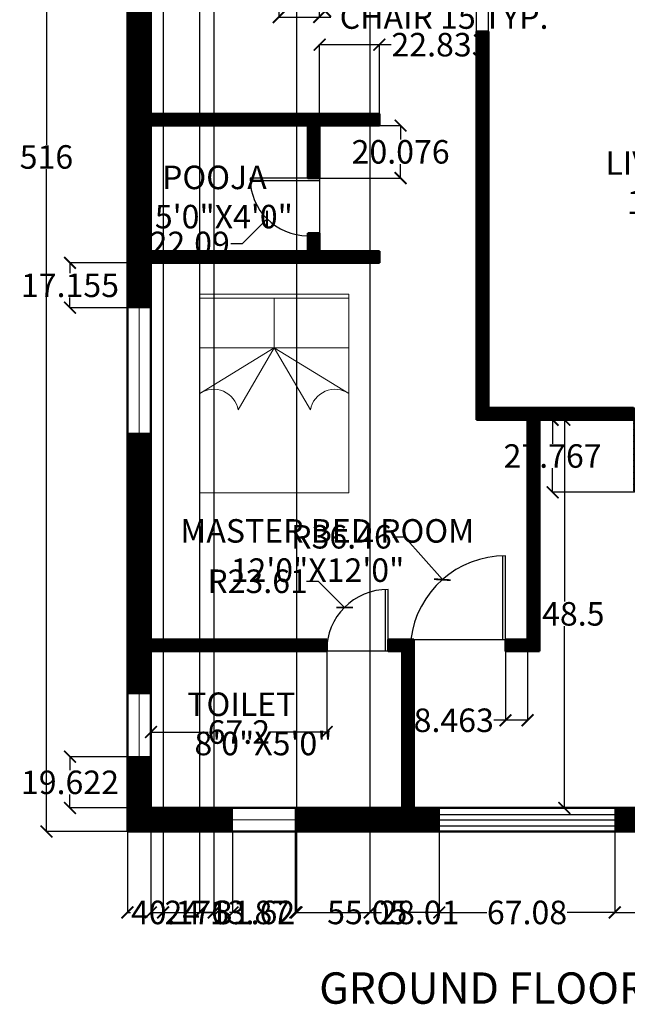
# Model space of a CAD drawing. Units: inches. Extents: x 91 to 526, y 242 to 861.
# Tile 1 of 5: x 96 to 328, y 242 to 618. Entities that reach past the tile are written whole.
import ezdxf

# ---------------------------------------------------------------- set-up
doc = ezdxf.new("R2010")
doc.units = ezdxf.units.IN
doc.header["$MEASUREMENT"] = 0
for name, color, linetype, lineweight in [('A-ANNO-DIMS', 2, 'Continuous', 18), ('A-ANNO-TEXT', 7, 'Continuous', 35), ('A-AREA-IDEN', 7, 'Continuous', 18), ('A-DOOR', 3, 'Continuous', 25), ('A-FLOR-STRS', 7, 'Continuous', 25), ('A-FURN', 8, 'Continuous', 18), ('A-GLAZ', 4, 'Continuous', 18), ('A-WALL', 7, 'Continuous', 50), ('A-WALL-PATT', 252, 'Continuous', 13)]:
    doc.layers.add(name, color=color, linetype=linetype, lineweight=lineweight)
doc.styles.get("Standard").update_dxf_attribs({"font": 'arial.ttf'})
doc.dimstyles.get("Standard").update_dxf_attribs({"dimtxt": 9, "dimasz": 4.5, "dimexe": 0.18, "dimexo": 0.0625, "dimgap": 0.09, "dimtad": 0, "dimtih": 1, "dimtoh": 1, "dimdec": 1, "dimzin": 0, "dimdsep": 46, "dimlunit": 4, "dimtxsty": 'Standard', "dimblk": 'ARCHTICK', "dimcen": 0.09, "dimadec": 0, "dimazin": 0, "dimtfac": 1, "dimtdec": 1, "dimtofl": 0, "dimtmove": 0, "dimatfit": 3, "dimfxl": 1, "dimtolj": 1, "dimtzin": 0, "dimarcsym": 0})

# ---------------------------------------------------------------- blocks, each defined once
blk = doc.blocks.new('WIN-48')
for p, q in [((0, 9), (48, 9)), ((0, 0), (0, 9)), ((48, 9), (48, 0)), ((0, 4.5), (48, 4.5)), ((48, 0), (0, 0))]:
    blk.add_line(p, q)
blk = doc.blocks.new('WIN-24')
for p, q in [((0, 24), (9, 24)), ((0, 0), (0, 24)), ((4.5, 0), (4.5, 24)), ((9, 24), (9, 0)), ((0, 0), (9, 0))]:
    blk.add_line(p, q)
blk = doc.blocks.new('BED-DOUBLE')
for p, q in [((0, 76.05), (57.04, 76.05)), ((0, 0), (0, 76.05)), ((57.04, 76.05), (57.04, 0)), ((0, 74.47), (57.04, 74.47)), ((28.52, 55.46), (28.52, 74.47)), ((0, 55.46), (57.04, 55.46)), ((28.52, 55.46), (0, 38.03)), ((14.73, 31.74), (28.52, 55.46)), ((57.04, 38.03), (28.52, 55.46)), ((28.52, 55.46), (42.31, 31.74)), ((57.04, 0), (0, 0))]:
    blk.add_line(p, q)
for centre, start, end in [((5.32, 30.09), 9.9572, 123.8152), ((51.72, 30.09), 56.1848, 170.0428)]:
    blk.add_arc(centre, 9.56, start, end)
blk = doc.blocks.new('_ArchTick')
at = {"color": 0, "linetype": 'ByBlock', "const_width": 0.15}
blk.add_lwpolyline([(-0.5, -0.5), (0.5, 0.5)], dxfattribs=at)
blk = doc.blocks.new('*D13')
at = {"layer": 'A-ANNO-DIMS', "color": 0, "lineweight": -2, "transparency": 16777216}
for p, q in [((195.04, 621.43), (195.04, 619)), ((210.48, 621.43), (210.48, 619)), ((195.04, 619.18), (210.48, 619.18)), ((210.48, 619.18), (214.98, 619.18))]:
    blk.add_line(p, q, dxfattribs=at)
at = {"layer": 'Defpoints', "color": 0, "transparency": 16777216}
for p in [(195.04, 621.5), (210.48, 621.5), (210.48, 619.18)]:
    blk.add_point(p, dxfattribs=at)
at = {"layer": 'A-ANNO-DIMS', "color": 0, "lineweight": -2, "transparency": 16777216, "xscale": 4.5, "yscale": 4.5, "zscale": 4.5, "rotation": 180}
blk.add_blockref('_ArchTick', (195.04, 619.18), dxfattribs=at)
at = {"layer": 'A-ANNO-DIMS', "color": 0, "lineweight": -2, "transparency": 16777216, "xscale": 4.5, "yscale": 4.5, "zscale": 4.5}
blk.add_blockref('_ArchTick', (210.48, 619.18), dxfattribs=at)
at = {"layer": 'A-ANNO-DIMS', "color": 0, "transparency": 16777216, "insert": (258.22, 619.18), "char_height": 9, "attachment_point": 5}
blk.add_mtext('\\A1;CHAIR 15 TYP.', dxfattribs=at)
blk = doc.blocks.new('*D14')
at = {"layer": 'A-ANNO-DIMS', "color": 0, "lineweight": -2, "transparency": 16777216}
for p, q in [((210.54, 631.24), (212.97, 631.24)), ((212.79, 631.24), (212.79, 631.05)), ((210.54, 621.5), (212.97, 621.5)), ((212.79, 621.5), (212.79, 621.68))]:
    blk.add_line(p, q, dxfattribs=at)
at = {"layer": 'Defpoints', "color": 0, "transparency": 16777216}
for p in [(210.48, 631.24), (212.79, 631.24), (210.48, 621.5)]:
    blk.add_point(p, dxfattribs=at)
at = {"layer": 'A-ANNO-DIMS', "color": 0, "lineweight": -2, "transparency": 16777216, "xscale": 4.5, "yscale": 4.5, "zscale": 4.5}
for p, rotation in [((212.79, 631.24), 90), ((212.79, 621.5), 270)]:
    blk.add_blockref('_ArchTick', p, dxfattribs=dict(at, rotation=rotation))
at = {"layer": 'A-ANNO-DIMS', "color": 0, "transparency": 16777216, "insert": (212.79, 626.37), "char_height": 9, "attachment_point": 5}
blk.add_mtext('\\A1;10 TYP.', dxfattribs=at)
blk = doc.blocks.new('*D18')
at = {"layer": 'A-ANNO-DIMS', "color": 0, "lineweight": -2, "transparency": 16777216}
for p, q in [((137.1, 823.67), (106.03, 823.67)), ((106.21, 823.67), (106.21, 570.36)), ((106.21, 307.67), (106.21, 560.99)), ((137.1, 307.67), (106.03, 307.67))]:
    blk.add_line(p, q, dxfattribs=at)
at = {"layer": 'Defpoints', "color": 0, "transparency": 16777216}
for p in [(106.21, 823.67), (137.16, 823.67), (137.16, 307.67)]:
    blk.add_point(p, dxfattribs=at)
at = {"layer": 'A-ANNO-DIMS', "color": 0, "lineweight": -2, "transparency": 16777216, "xscale": 4.5, "yscale": 4.5, "zscale": 4.5}
for p, rotation in [((106.21, 823.67), 90), ((106.21, 307.67), 270)]:
    blk.add_blockref('_ArchTick', p, dxfattribs=dict(at, rotation=rotation))
at = {"layer": 'A-ANNO-DIMS', "color": 0, "transparency": 16777216, "insert": (106.21, 565.67), "char_height": 9, "attachment_point": 5}
blk.add_mtext('\\A1;516', dxfattribs=at)
blk = doc.blocks.new('*D22')
at = {"layer": 'A-ANNO-DIMS', "color": 0, "lineweight": -2, "transparency": 16777216}
for p, q in [((137.16, 307.61), (137.16, 276.54)), ((177.34, 307.61), (177.34, 276.54)), ((137.16, 276.72), (138.3, 276.72)), ((177.34, 276.72), (176.2, 276.72))]:
    blk.add_line(p, q, dxfattribs=at)
at = {"layer": 'Defpoints', "color": 0, "transparency": 16777216}
for p in [(137.16, 307.67), (177.34, 307.67), (177.34, 276.72)]:
    blk.add_point(p, dxfattribs=at)
at = {"layer": 'A-ANNO-DIMS', "color": 0, "lineweight": -2, "transparency": 16777216, "xscale": 4.5, "yscale": 4.5, "zscale": 4.5, "rotation": 180}
blk.add_blockref('_ArchTick', (137.16, 276.72), dxfattribs=at)
at = {"layer": 'A-ANNO-DIMS', "color": 0, "lineweight": -2, "transparency": 16777216, "xscale": 4.5, "yscale": 4.5, "zscale": 4.5}
blk.add_blockref('_ArchTick', (177.34, 276.72), dxfattribs=at)
at = {"layer": 'A-ANNO-DIMS', "color": 0, "transparency": 16777216, "insert": (157.25, 276.72), "char_height": 9, "attachment_point": 5}
blk.add_mtext('\\A1;40.176', dxfattribs=at)
blk = doc.blocks.new('*D23')
at = {"layer": 'A-ANNO-DIMS', "color": 0, "lineweight": -2, "transparency": 16777216}
for p, q in [((201.34, 307.61), (201.34, 276.54)), ((256.39, 307.61), (256.39, 276.54)), ((201.34, 276.72), (213.55, 276.72)), ((256.39, 276.72), (244.17, 276.72))]:
    blk.add_line(p, q, dxfattribs=at)
at = {"layer": 'Defpoints', "color": 0, "transparency": 16777216}
for p in [(201.34, 307.67), (256.39, 307.67), (256.39, 276.72)]:
    blk.add_point(p, dxfattribs=at)
at = {"layer": 'A-ANNO-DIMS', "color": 0, "lineweight": -2, "transparency": 16777216, "xscale": 4.5, "yscale": 4.5, "zscale": 4.5, "rotation": 180}
blk.add_blockref('_ArchTick', (201.34, 276.72), dxfattribs=at)
at = {"layer": 'A-ANNO-DIMS', "color": 0, "lineweight": -2, "transparency": 16777216, "xscale": 4.5, "yscale": 4.5, "zscale": 4.5}
blk.add_blockref('_ArchTick', (256.39, 276.72), dxfattribs=at)
at = {"layer": 'A-ANNO-DIMS', "color": 0, "transparency": 16777216, "insert": (228.86, 276.72), "char_height": 9, "attachment_point": 5}
blk.add_mtext('\\A1;55.05', dxfattribs=at)
blk = doc.blocks.new('*D24')
at = {"layer": 'A-ANNO-DIMS', "color": 0, "lineweight": -2, "transparency": 16777216}
for p, q in [((256.39, 307.61), (256.39, 276.54)), ((323.47, 307.61), (323.47, 276.54)), ((256.39, 276.72), (274.62, 276.72)), ((323.47, 276.72), (305.24, 276.72))]:
    blk.add_line(p, q, dxfattribs=at)
at = {"layer": 'Defpoints', "color": 0, "transparency": 16777216}
for p in [(256.39, 307.67), (323.47, 307.67), (323.47, 276.72)]:
    blk.add_point(p, dxfattribs=at)
at = {"layer": 'A-ANNO-DIMS', "color": 0, "lineweight": -2, "transparency": 16777216, "xscale": 4.5, "yscale": 4.5, "zscale": 4.5, "rotation": 180}
blk.add_blockref('_ArchTick', (256.39, 276.72), dxfattribs=at)
at = {"layer": 'A-ANNO-DIMS', "color": 0, "lineweight": -2, "transparency": 16777216, "xscale": 4.5, "yscale": 4.5, "zscale": 4.5}
blk.add_blockref('_ArchTick', (323.47, 276.72), dxfattribs=at)
at = {"layer": 'A-ANNO-DIMS', "color": 0, "transparency": 16777216, "insert": (289.93, 276.72), "char_height": 9, "attachment_point": 5}
blk.add_mtext('\\A1;67.08', dxfattribs=at)
blk = doc.blocks.new('*D25')
at = {"layer": 'A-ANNO-DIMS', "color": 0, "lineweight": -2, "transparency": 16777216}
for p, q in [((323.47, 307.61), (323.47, 276.54)), ((393.61, 307.61), (393.61, 276.54)), ((323.47, 276.72), (343.32, 276.72)), ((393.61, 276.72), (373.76, 276.72))]:
    blk.add_line(p, q, dxfattribs=at)
at = {"layer": 'Defpoints', "color": 0, "transparency": 16777216}
for p in [(323.47, 307.67), (393.61, 307.67), (393.61, 276.72)]:
    blk.add_point(p, dxfattribs=at)
at = {"layer": 'A-ANNO-DIMS', "color": 0, "lineweight": -2, "transparency": 16777216, "xscale": 4.5, "yscale": 4.5, "zscale": 4.5, "rotation": 180}
blk.add_blockref('_ArchTick', (323.47, 276.72), dxfattribs=at)
at = {"layer": 'A-ANNO-DIMS', "color": 0, "lineweight": -2, "transparency": 16777216, "xscale": 4.5, "yscale": 4.5, "zscale": 4.5}
blk.add_blockref('_ArchTick', (393.61, 276.72), dxfattribs=at)
at = {"layer": 'A-ANNO-DIMS', "color": 0, "transparency": 16777216, "insert": (358.54, 276.72), "char_height": 9, "attachment_point": 5}
blk.add_mtext('\\A1;70.14', dxfattribs=at)
blk = doc.blocks.new('*D26')
at = {"layer": 'A-ANNO-DIMS', "color": 0, "lineweight": -2, "transparency": 16777216}
for p, q in [((146.1, 336.29), (115.03, 336.29)), ((115.21, 336.29), (115.21, 331.17)), ((115.21, 316.67), (115.21, 321.8)), ((146.1, 316.67), (115.03, 316.67))]:
    blk.add_line(p, q, dxfattribs=at)
at = {"layer": 'Defpoints', "color": 0, "transparency": 16777216}
for p in [(115.21, 336.29), (146.16, 336.29), (146.16, 316.67)]:
    blk.add_point(p, dxfattribs=at)
at = {"layer": 'A-ANNO-DIMS', "color": 0, "lineweight": -2, "transparency": 16777216, "xscale": 4.5, "yscale": 4.5, "zscale": 4.5}
for p, rotation in [((115.21, 336.29), 90), ((115.21, 316.67), 270)]:
    blk.add_blockref('_ArchTick', p, dxfattribs=dict(at, rotation=rotation))
at = {"layer": 'A-ANNO-DIMS', "color": 0, "transparency": 16777216, "insert": (115.21, 326.48), "char_height": 9, "attachment_point": 5}
blk.add_mtext('\\A1;19.622', dxfattribs=at)
blk = doc.blocks.new('*D27')
at = {"layer": 'A-ANNO-DIMS', "color": 0, "lineweight": -2, "transparency": 16777216}
for p, q in [((146.1, 525.17), (115.03, 525.17)), ((115.21, 525.17), (115.21, 521.28)), ((115.21, 508.02), (115.21, 511.91)), ((146.1, 508.02), (115.03, 508.02))]:
    blk.add_line(p, q, dxfattribs=at)
at = {"layer": 'Defpoints', "color": 0, "transparency": 16777216}
for p in [(115.21, 525.17), (146.16, 525.17), (146.16, 508.02)]:
    blk.add_point(p, dxfattribs=at)
at = {"layer": 'A-ANNO-DIMS', "color": 0, "lineweight": -2, "transparency": 16777216, "xscale": 4.5, "yscale": 4.5, "zscale": 4.5}
for p, rotation in [((115.21, 525.17), 90), ((115.21, 508.02), 270)]:
    blk.add_blockref('_ArchTick', p, dxfattribs=dict(at, rotation=rotation))
at = {"layer": 'A-ANNO-DIMS', "color": 0, "transparency": 16777216, "insert": (115.21, 516.59), "char_height": 9, "attachment_point": 5}
blk.add_mtext('\\A1;17.155', dxfattribs=at)
blk = doc.blocks.new('*D35')
at = {"layer": 'A-ANNO-DIMS', "color": 0, "lineweight": -2, "transparency": 16777216}
for p, q in [((335.1, 465.17), (304.03, 465.17)), ((304.21, 465.17), (304.21, 395.61)), ((304.21, 316.67), (304.21, 386.24)), ((335.1, 316.67), (304.03, 316.67))]:
    blk.add_line(p, q, dxfattribs=at)
at = {"layer": 'Defpoints', "color": 0, "transparency": 16777216}
for p in [(304.21, 465.17), (335.16, 465.17), (335.16, 316.67)]:
    blk.add_point(p, dxfattribs=at)
at = {"layer": 'A-ANNO-DIMS', "color": 0, "lineweight": -2, "transparency": 16777216, "xscale": 4.5, "yscale": 4.5, "zscale": 4.5}
for p, rotation in [((304.21, 465.17), 90), ((304.21, 316.67), 270)]:
    blk.add_blockref('_ArchTick', p, dxfattribs=dict(at, rotation=rotation))
at = {"layer": 'A-ANNO-DIMS', "color": 0, "transparency": 16777216, "insert": (304.21, 390.92), "char_height": 9, "attachment_point": 5}
blk.add_mtext('\\A1;148.5', dxfattribs=at)
blk = doc.blocks.new('*D36')
at = {"layer": 'A-ANNO-DIMS', "color": 0, "lineweight": -2, "transparency": 16777216}
for p, q in [((270.66, 613.73), (270.66, 644.8)), ((270.66, 644.62), (275.16, 644.62)), ((275.16, 613.73), (275.16, 644.8)), ((275.16, 644.62), (279.66, 644.62))]:
    blk.add_line(p, q, dxfattribs=at)
at = {"layer": 'Defpoints', "color": 0, "transparency": 16777216}
for p in [(275.16, 644.62), (270.66, 613.67), (275.16, 613.67)]:
    blk.add_point(p, dxfattribs=at)
at = {"layer": 'A-ANNO-DIMS', "color": 0, "lineweight": -2, "transparency": 16777216, "xscale": 4.5, "yscale": 4.5, "zscale": 4.5, "rotation": 180}
blk.add_blockref('_ArchTick', (270.66, 644.62), dxfattribs=at)
at = {"layer": 'A-ANNO-DIMS', "color": 0, "lineweight": -2, "transparency": 16777216, "xscale": 4.5, "yscale": 4.5, "zscale": 4.5}
blk.add_blockref('_ArchTick', (275.16, 644.62), dxfattribs=at)
at = {"layer": 'A-ANNO-DIMS', "color": 0, "transparency": 16777216, "insert": (288.16, 644.62), "char_height": 9, "attachment_point": 5}
blk.add_mtext('\\A1;4.5', dxfattribs=at)
blk = doc.blocks.new('*D38')
at = {"layer": 'A-ANNO-DIMS', "color": 0, "lineweight": -2, "transparency": 16777216}
for p, q in [((146.16, 718.61), (146.16, 276.54)), ((170.16, 718.61), (170.16, 276.54)), ((146.16, 276.72), (151.57, 276.72)), ((170.16, 276.72), (164.75, 276.72))]:
    blk.add_line(p, q, dxfattribs=at)
at = {"layer": 'Defpoints', "color": 0, "transparency": 16777216}
for p in [(146.16, 718.67), (170.16, 718.67), (170.16, 276.72)]:
    blk.add_point(p, dxfattribs=at)
at = {"layer": 'A-ANNO-DIMS', "color": 0, "lineweight": -2, "transparency": 16777216, "xscale": 4.5, "yscale": 4.5, "zscale": 4.5, "rotation": 180}
blk.add_blockref('_ArchTick', (146.16, 276.72), dxfattribs=at)
at = {"layer": 'A-ANNO-DIMS', "color": 0, "lineweight": -2, "transparency": 16777216, "xscale": 4.5, "yscale": 4.5, "zscale": 4.5}
blk.add_blockref('_ArchTick', (170.16, 276.72), dxfattribs=at)
at = {"layer": 'A-ANNO-DIMS', "color": 0, "transparency": 16777216, "insert": (158.16, 276.72), "char_height": 9, "attachment_point": 5}
blk.add_mtext('\\A1;24', dxfattribs=at)
blk = doc.blocks.new('*D39')
at = {"layer": 'A-ANNO-DIMS', "color": 0, "lineweight": -2, "transparency": 16777216}
for p, q in [((201.78, 794.78), (201.78, 276.54)), ((229.79, 794.78), (229.79, 276.54)), ((201.78, 276.72), (229.79, 276.72)), ((229.79, 276.72), (234.29, 276.72))]:
    blk.add_line(p, q, dxfattribs=at)
at = {"layer": 'Defpoints', "color": 0, "transparency": 16777216}
for p in [(201.78, 794.84), (229.79, 794.84), (229.79, 276.72)]:
    blk.add_point(p, dxfattribs=at)
at = {"layer": 'A-ANNO-DIMS', "color": 0, "lineweight": -2, "transparency": 16777216, "xscale": 4.5, "yscale": 4.5, "zscale": 4.5, "rotation": 180}
blk.add_blockref('_ArchTick', (201.78, 276.72), dxfattribs=at)
at = {"layer": 'A-ANNO-DIMS', "color": 0, "lineweight": -2, "transparency": 16777216, "xscale": 4.5, "yscale": 4.5, "zscale": 4.5}
blk.add_blockref('_ArchTick', (229.79, 276.72), dxfattribs=at)
at = {"layer": 'A-ANNO-DIMS', "color": 0, "transparency": 16777216, "insert": (248.77, 276.72), "char_height": 9, "attachment_point": 5}
blk.add_mtext('\\A1;28.01', dxfattribs=at)
blk = doc.blocks.new('*D41')
at = {"layer": 'A-ANNO-DIMS', "color": 0, "lineweight": -2, "transparency": 16777216}
for p, q in [((150.78, 748.14), (150.78, 276.54)), ((164.66, 748.14), (164.66, 276.54)), ((150.78, 276.72), (164.66, 276.72)), ((164.66, 276.72), (169.16, 276.72))]:
    blk.add_line(p, q, dxfattribs=at)
at = {"layer": 'Defpoints', "color": 0, "transparency": 16777216}
for p in [(150.78, 748.2), (164.66, 748.2), (164.66, 276.72)]:
    blk.add_point(p, dxfattribs=at)
at = {"layer": 'A-ANNO-DIMS', "color": 0, "lineweight": -2, "transparency": 16777216, "xscale": 4.5, "yscale": 4.5, "zscale": 4.5, "rotation": 180}
blk.add_blockref('_ArchTick', (150.78, 276.72), dxfattribs=at)
at = {"layer": 'A-ANNO-DIMS', "color": 0, "lineweight": -2, "transparency": 16777216, "xscale": 4.5, "yscale": 4.5, "zscale": 4.5}
blk.add_blockref('_ArchTick', (164.66, 276.72), dxfattribs=at)
at = {"layer": 'A-ANNO-DIMS', "color": 0, "transparency": 16777216, "insert": (184.01, 276.72), "char_height": 9, "attachment_point": 5}
blk.add_mtext('\\A1;13.87', dxfattribs=at)
blk = doc.blocks.new('*D44')
at = {"layer": 'A-ANNO-DIMS', "color": 0, "lineweight": -2, "transparency": 16777216}
for p, q in [((201.78, 794.78), (201.78, 276.54)), ((170.16, 790.61), (170.16, 276.54)), ((170.16, 276.72), (170.74, 276.72)), ((201.78, 276.72), (201.2, 276.72))]:
    blk.add_line(p, q, dxfattribs=at)
at = {"layer": 'Defpoints', "color": 0, "transparency": 16777216}
for p in [(201.78, 794.84), (170.16, 790.67), (201.78, 276.72)]:
    blk.add_point(p, dxfattribs=at)
at = {"layer": 'A-ANNO-DIMS', "color": 0, "lineweight": -2, "transparency": 16777216, "xscale": 4.5, "yscale": 4.5, "zscale": 4.5, "rotation": 180}
blk.add_blockref('_ArchTick', (170.16, 276.72), dxfattribs=at)
at = {"layer": 'A-ANNO-DIMS', "color": 0, "lineweight": -2, "transparency": 16777216, "xscale": 4.5, "yscale": 4.5, "zscale": 4.5}
blk.add_blockref('_ArchTick', (201.78, 276.72), dxfattribs=at)
at = {"layer": 'A-ANNO-DIMS', "color": 0, "transparency": 16777216, "insert": (185.97, 276.72), "char_height": 9, "attachment_point": 5}
blk.add_mtext('\\A1;31.62', dxfattribs=at)
blk = doc.blocks.new('*D48')
at = {"layer": 'A-ANNO-DIMS', "color": 0, "lineweight": -2, "transparency": 16777216}
for p, q in [((146.16, 376.61), (146.16, 345.54)), ((213.35, 376.61), (213.35, 345.54)), ((146.16, 345.72), (168, 345.72)), ((213.35, 345.72), (191.51, 345.72))]:
    blk.add_line(p, q, dxfattribs=at)
at = {"layer": 'Defpoints', "color": 0, "transparency": 16777216}
for p in [(146.16, 376.67), (213.35, 376.67), (146.16, 345.72)]:
    blk.add_point(p, dxfattribs=at)
at = {"layer": 'A-ANNO-DIMS', "color": 0, "lineweight": -2, "transparency": 16777216, "xscale": 4.5, "yscale": 4.5, "zscale": 4.5}
for p, rotation in [((146.16, 345.72), 179.9999999999999), ((213.35, 345.72), 359.9999999999999)]:
    blk.add_blockref('_ArchTick', p, dxfattribs=dict(at, rotation=rotation))
at = {"layer": 'A-ANNO-DIMS', "color": 0, "transparency": 16777216, "insert": (179.76, 345.72), "char_height": 9, "attachment_point": 5}
blk.add_mtext('\\A1;67.2', dxfattribs=at)
blk = doc.blocks.new('*D49')
at = {"layer": 'A-ANNO-DIMS', "color": 0, "lineweight": -2, "transparency": 16777216}
for p, q in [((281.7, 381.11), (281.7, 350.04)), ((290.16, 381.11), (290.16, 350.04)), ((281.7, 350.22), (277.2, 350.22)), ((290.16, 350.22), (281.7, 350.22))]:
    blk.add_line(p, q, dxfattribs=at)
at = {"layer": 'Defpoints', "color": 0, "transparency": 16777216}
for p in [(281.7, 381.17), (290.16, 381.17), (281.7, 350.22)]:
    blk.add_point(p, dxfattribs=at)
at = {"layer": 'A-ANNO-DIMS', "color": 0, "lineweight": -2, "transparency": 16777216, "xscale": 4.5, "yscale": 4.5, "zscale": 4.5, "rotation": 180}
blk.add_blockref('_ArchTick', (281.7, 350.22), dxfattribs=at)
at = {"layer": 'A-ANNO-DIMS', "color": 0, "lineweight": -2, "transparency": 16777216, "xscale": 4.5, "yscale": 4.5, "zscale": 4.5}
blk.add_blockref('_ArchTick', (290.16, 350.22), dxfattribs=at)
at = {"layer": 'A-ANNO-DIMS', "color": 0, "transparency": 16777216, "insert": (261.92, 350.22), "char_height": 9, "attachment_point": 5}
blk.add_mtext('\\A1;8.463', dxfattribs=at)
blk = doc.blocks.new('*D50')
at = {"layer": 'A-ANNO-DIMS', "color": 0, "lineweight": -2, "transparency": 16777216}
for p, q in [((330.6, 465.17), (299.53, 465.17)), ((299.71, 465.17), (299.71, 455.97)), ((299.71, 437.4), (299.71, 446.6)), ((330.6, 437.4), (299.53, 437.4))]:
    blk.add_line(p, q, dxfattribs=at)
at = {"layer": 'Defpoints', "color": 0, "transparency": 16777216}
for p in [(299.71, 465.17), (330.66, 465.17), (330.66, 437.4)]:
    blk.add_point(p, dxfattribs=at)
at = {"layer": 'A-ANNO-DIMS', "color": 0, "lineweight": -2, "transparency": 16777216, "xscale": 4.5, "yscale": 4.5, "zscale": 4.5}
for p, rotation in [((299.71, 465.17), 90), ((299.71, 437.4), 270)]:
    blk.add_blockref('_ArchTick', p, dxfattribs=dict(at, rotation=rotation))
at = {"layer": 'A-ANNO-DIMS', "color": 0, "transparency": 16777216, "insert": (299.71, 451.29), "char_height": 9, "attachment_point": 5}
blk.add_mtext('\\A1;27.767', dxfattribs=at)
blk = doc.blocks.new('*D52')
at = {"layer": 'A-ANNO-DIMS', "color": 0, "lineweight": -2, "transparency": 16777216}
for p, q in [((210.72, 577.67), (241.79, 577.67)), ((241.61, 577.67), (241.61, 572.32)), ((241.61, 557.6), (241.61, 562.95)), ((210.72, 557.6), (241.79, 557.6))]:
    blk.add_line(p, q, dxfattribs=at)
at = {"layer": 'Defpoints', "color": 0, "transparency": 16777216}
for p in [(210.66, 577.67), (210.66, 557.6), (241.61, 557.6)]:
    blk.add_point(p, dxfattribs=at)
at = {"layer": 'A-ANNO-DIMS', "color": 0, "lineweight": -2, "transparency": 16777216, "xscale": 4.5, "yscale": 4.5, "zscale": 4.5}
for p, rotation in [((241.61, 577.67), 90), ((241.61, 557.6), 270)]:
    blk.add_blockref('_ArchTick', p, dxfattribs=dict(at, rotation=rotation))
at = {"layer": 'A-ANNO-DIMS', "color": 0, "transparency": 16777216, "insert": (241.61, 567.63), "char_height": 9, "attachment_point": 5}
blk.add_mtext('\\A1;20.076', dxfattribs=at)
blk = doc.blocks.new('*D55')
at = {"layer": 'A-ANNO-DIMS', "color": 0, "lineweight": -2, "transparency": 16777216}
for p, q in [((210.66, 577.73), (210.66, 608.8)), ((210.66, 608.62), (233.49, 608.62)), ((233.49, 577.73), (233.49, 608.8)), ((233.49, 608.62), (237.99, 608.62))]:
    blk.add_line(p, q, dxfattribs=at)
at = {"layer": 'Defpoints', "color": 0, "transparency": 16777216}
for p in [(233.49, 608.62), (210.66, 577.67), (233.49, 577.67)]:
    blk.add_point(p, dxfattribs=at)
at = {"layer": 'A-ANNO-DIMS', "color": 0, "lineweight": -2, "transparency": 16777216, "xscale": 4.5, "yscale": 4.5, "zscale": 4.5, "rotation": 180}
blk.add_blockref('_ArchTick', (210.66, 608.62), dxfattribs=at)
at = {"layer": 'A-ANNO-DIMS', "color": 0, "lineweight": -2, "transparency": 16777216, "xscale": 4.5, "yscale": 4.5, "zscale": 4.5}
blk.add_blockref('_ArchTick', (233.49, 608.62), dxfattribs=at)
at = {"layer": 'A-ANNO-DIMS', "color": 0, "transparency": 16777216, "insert": (256.84, 608.62), "char_height": 9, "attachment_point": 5}
blk.add_mtext('\\A1;22.833', dxfattribs=at)
blk = doc.blocks.new('*D59')
at = {"layer": 'A-ANNO-DIMS', "color": 0, "lineweight": -2, "transparency": 16777216}
for p, q in [((238.57, 420.4), (243.07, 420.4)), ((243.07, 420.4), (257.56, 404)), ((281.61, 376.67), (281.79, 376.67)), ((281.7, 376.58), (281.7, 376.76))]:
    blk.add_line(p, q, dxfattribs=at)
at = {"layer": 'Defpoints', "color": 0, "transparency": 16777216}
for p in [(257.56, 404), (281.7, 376.67)]:
    blk.add_point(p, dxfattribs=at)
at = {"layer": 'A-ANNO-DIMS', "color": 0, "lineweight": -2, "transparency": 16777216, "xscale": 4.5, "yscale": 4.5, "zscale": 4.5, "rotation": 311.4548896463722}
blk.add_blockref('_ArchTick', (257.56, 404), dxfattribs=at)
at = {"layer": 'A-ANNO-DIMS', "color": 0, "transparency": 16777216, "insert": (219, 420.4), "char_height": 9, "attachment_point": 5}
blk.add_mtext('\\A1;R36.46', dxfattribs=at)
blk = doc.blocks.new('*D64')
at = {"layer": 'A-ANNO-DIMS', "color": 0, "lineweight": -2, "transparency": 16777216}
for p, q in [((205.64, 403.39), (210.14, 403.39)), ((210.14, 403.39), (220.16, 393.37)), ((236.77, 376.67), (236.95, 376.67)), ((236.86, 376.58), (236.86, 376.76))]:
    blk.add_line(p, q, dxfattribs=at)
at = {"layer": 'Defpoints', "color": 0, "transparency": 16777216}
for p in [(220.16, 393.37), (236.86, 376.67)]:
    blk.add_point(p, dxfattribs=at)
at = {"layer": 'A-ANNO-DIMS', "color": 0, "lineweight": -2, "transparency": 16777216, "xscale": 4.5, "yscale": 4.5, "zscale": 4.5, "rotation": 314.9988795521384}
blk.add_blockref('_ArchTick', (220.16, 393.37), dxfattribs=at)
at = {"layer": 'A-ANNO-DIMS', "color": 0, "transparency": 16777216, "insert": (186.93, 403.39), "char_height": 9, "attachment_point": 5}
blk.add_mtext('\\A1;R23.61', dxfattribs=at)
blk = doc.blocks.new('*D65')
at = {"layer": 'A-ANNO-DIMS', "color": 0, "lineweight": -2, "transparency": 16777216}
for p, q in [((206.07, 557.6), (206.25, 557.6)), ((206.16, 557.51), (206.16, 557.69)), ((181.17, 532.6), (190.54, 541.98)), ((176.67, 532.6), (181.17, 532.6))]:
    blk.add_line(p, q, dxfattribs=at)
at = {"layer": 'Defpoints', "color": 0, "transparency": 16777216}
for p in [(206.16, 557.6), (190.54, 541.98)]:
    blk.add_point(p, dxfattribs=at)
at = {"layer": 'A-ANNO-DIMS', "color": 0, "lineweight": -2, "transparency": 16777216, "xscale": 4.5, "yscale": 4.5, "zscale": 4.5, "rotation": 44.99971205687489}
blk.add_blockref('_ArchTick', (190.54, 541.98), dxfattribs=at)
at = {"layer": 'A-ANNO-DIMS', "color": 0, "transparency": 16777216, "insert": (157.08, 532.6), "char_height": 9, "attachment_point": 5}
blk.add_mtext('\\A1;R22.09', dxfattribs=at)

msp = doc.modelspace()

# ---------------------------------------------------------------- hatches: boundary and pattern name
at = {"layer": 'A-WALL-PATT'}
h = msp.add_hatch(dxfattribs=at)
h.set_pattern_fill('ANSI31', color=256)
h.paths.add_polyline_path([(476.1605, 544.131), (467.1605, 544.131), (467.1605, 469.6714), (381.2784, 469.6714), (381.2784, 467.1295, -0.01443214), (381.4527, 465.1714), (467.1605, 465.1714), (467.1605, 417.4774), (476.1605, 417.4774)])
h.paths.add_polyline_path([(476.1605, 637.294), (467.1605, 637.294), (467.1605, 618.1714), (383.1605, 618.1714), (383.1605, 650.6481), (381.8098, 650.6481, -0.04281846), (378.6605, 650.378), (378.6605, 618.1714), (378.6605, 613.6714), (467.1605, 613.6714), (467.1605, 592.131), (476.1605, 592.131)])
h.paths.add_polyline_path([(476.1605, 699.6337), (467.1605, 699.6337), (467.1605, 682.6714), (378.6605, 682.6714), (367.8126, 682.6714), (367.8126, 678.1714), (378.6605, 678.1714), (378.6605, 668.8665), (383.1605, 668.8665), (383.1605, 678.1714), (467.1605, 678.1714), (467.1605, 661.294), (476.1605, 661.294)])
h.paths.add_polyline_path([(476.1605, 823.6714), (423.2305, 823.6714), (423.2305, 814.6714), (467.1605, 814.6714), (467.1605, 747.6337), (476.1605, 747.6337)])
h.paths.add_polyline_path([(375.2305, 823.6714), (311.1029, 823.6714), (311.1029, 814.6714), (330.6605, 814.6714), (330.6605, 682.6714), (335.1605, 682.6714), (335.1605, 814.6714), (375.2305, 814.6714)])
h.paths.add_polyline_path([(287.1029, 823.6714), (230.7133, 823.6714), (230.7133, 814.6714), (266.1605, 814.6714), (266.1605, 755.4247), (270.6605, 755.4247), (270.6605, 814.6714), (287.1029, 814.6714)])
h.paths.add_polyline_path([(182.7133, 823.6714), (137.1605, 823.6714), (137.1605, 675.6513), (146.1605, 675.6513), (146.1605, 714.1714), (178.4758, 714.1714), (178.4758, 718.6714), (146.1605, 718.6714), (146.1605, 814.6714), (182.7133, 814.6714)])
h.paths.add_polyline_path([(146.1605, 577.6714), (206.1605, 577.6714), (206.1605, 557.5953), (210.6605, 557.5953), (210.6605, 577.6714), (233.4933, 577.6714), (233.4933, 582.1714), (210.6605, 582.1714), (146.1605, 582.1714), (146.1605, 627.6513), (137.1605, 627.6513), (137.1605, 508.0167), (146.1605, 508.0167), (146.1605, 525.1714), (210.6605, 525.1714), (233.4933, 525.1714), (233.4933, 529.6714), (210.6605, 529.6714), (210.6605, 536.5826), (206.1605, 536.5826), (206.1605, 529.6714), (146.1605, 529.6714)])
h.paths.add_polyline_path([(146.1605, 460.0167), (137.1605, 460.0167), (137.1605, 360.2935), (146.1605, 360.2935), (146.1605, 376.6714), (210.6605, 376.6714), (213.2441, 376.6714, -0.02418169), (213.3544, 378.9513), (213.3544, 381.1714), (210.6605, 381.1714), (146.1605, 381.1714)])
h.paths.add_polyline_path([(146.1605, 336.2935), (137.1605, 336.2935), (137.1605, 307.6714), (146.1605, 307.6714), (177.3362, 307.6714), (177.3362, 316.6714), (146.1605, 316.6714)])
h.paths.add_polyline_path([(393.6086, 316.6714), (323.4726, 316.6714), (323.4726, 307.6714), (393.6086, 307.6714)])
h.paths.add_polyline_path([(256.39, 316.6714), (201.3362, 316.6714), (201.3362, 307.6714), (256.39, 307.6714)])
h.paths.add_polyline_path([(246.6605, 376.6714), (246.6605, 381.1714), (236.8559, 381.1714), (236.8559, 376.6714), (242.1605, 376.6714), (242.1605, 316.6714), (246.6605, 316.6714)])
h = msp.add_hatch(dxfattribs=at)
h.set_pattern_fill('ANSI31', color=256)
h.paths.add_polyline_path([(335.1605, 465.1714), (347.4545, 465.1714), (347.4545, 469.6714), (335.1605, 469.6714), (330.6605, 469.6714), (275.1605, 469.6714), (275.1605, 613.6714), (270.6605, 613.6714), (270.6605, 469.6714), (270.6605, 465.1714), (290.1605, 465.1714), (290.1605, 381.1714), (281.6979, 381.1714), (281.6979, 376.6714), (294.6605, 376.6714), (294.6605, 381.1714), (294.6605, 465.1714), (330.6605, 465.1714), (330.6605, 437.4043), (335.1605, 437.4043)])

# ---------------------------------------------------------------- linework, layer by layer
at = {"layer": 'A-DOOR'}
for p, q in [((210.6605, 557.5953), (184.0703, 557.5953)), ((210.6605, 557.5953), (210.6605, 535.9683)), ((210.6605, 556.5953), (184.0929, 556.5953)), ((280.6979, 381.1714), (280.6979, 413.1211)), ((281.6979, 381.1714), (281.6979, 413.1348)), ((235.8559, 376.6714), (235.8559, 400.2621)), ((236.8559, 376.6714), (236.8559, 400.2832)), ((246.6605, 381.1714), (281.6979, 381.1714)), ((236.8559, 376.6714), (213.2441, 376.6714))]:
    msp.add_line(p, q, dxfattribs=at)
for centre, radius, start, end in [((206.1605, 557.5953), 22.0902, 180, 270), ((281.6979, 376.6714), 36.4634, 90, 172.910966), ((236.8559, 376.6714), 23.6118, 90, 180)]:
    msp.add_arc(centre, radius, start, end, dxfattribs=at)
at = {"layer": 'A-FLOR-STRS'}
for p, q in [((256.39, 316.6714), (256.39, 307.6714)), ((323.4726, 316.6714), (323.4726, 307.6714)), ((256.39, 314.2283), (323.4726, 314.2283)), ((256.39, 312.1714), (323.4726, 312.1714)), ((256.39, 309.8425), (323.4726, 309.8425))]:
    msp.add_line(p, q, dxfattribs=at)
at = {"layer": 'A-WALL'}
for p, q in [((137.1605, 823.6714), (137.1605, 307.6714)), ((146.1605, 714.1714), (146.1605, 582.1714)), ((270.6605, 613.6714), (270.6605, 469.6714)), ((275.1605, 613.6714), (270.6605, 613.6714)), ((275.1605, 613.6714), (275.1605, 469.6714)), ((146.1605, 582.1714), (210.6605, 582.1714)), ((210.6605, 582.1714), (233.4933, 582.1714)), ((233.4933, 577.6714), (233.4933, 582.1714)), ((146.1605, 577.6714), (206.1605, 577.6714)), ((146.1605, 577.6714), (146.1605, 529.6714)), ((206.1605, 577.6714), (206.1605, 557.5953)), ((210.6605, 577.6714), (210.6605, 557.5953)), ((210.6605, 577.6714), (233.4933, 577.6714)), ((206.1605, 557.5953), (210.6605, 557.5953)), ((206.1605, 536.5826), (210.6605, 536.5826)), ((206.1605, 536.5826), (206.1605, 529.6714)), ((210.6605, 536.5826), (210.6605, 529.6714)), ((146.1605, 529.6714), (206.1605, 529.6714)), ((210.6605, 529.6714), (233.4933, 529.6714)), ((233.4933, 529.6714), (233.4933, 525.1714)), ((146.1605, 525.1714), (210.6605, 525.1714)), ((146.1605, 525.1714), (146.1605, 381.1714)), ((210.6605, 525.1714), (233.4933, 525.1714)), ((270.6605, 469.6714), (270.6605, 465.1714)), ((330.6605, 469.6714), (275.1605, 469.6714)), ((290.1605, 465.1714), (270.6605, 465.1714)), ((290.1605, 465.1714), (290.1605, 381.1714)), ((330.6605, 465.1714), (294.6605, 465.1714)), ((294.6605, 465.1714), (294.6605, 381.1714)), ((146.1605, 381.1714), (210.6605, 381.1714)), ((210.6605, 381.1714), (213.3544, 381.1714)), ((213.3544, 376.6714), (213.3544, 381.1714)), ((236.8559, 376.6714), (236.8559, 381.1714)), ((236.8559, 381.1714), (246.6605, 381.1714)), ((246.6605, 376.6714), (246.6605, 381.1714)), ((281.6979, 376.6714), (281.6979, 381.1714)), ((281.6979, 381.1714), (290.1605, 381.1714)), ((294.6605, 381.1714), (294.6605, 376.6714)), ((146.1605, 376.6714), (210.6605, 376.6714)), ((146.1605, 376.6714), (146.1605, 316.6714)), ((210.6605, 376.6714), (213.3544, 376.6714)), ((236.8559, 376.6714), (242.1605, 376.6714)), ((242.1605, 376.6714), (242.1605, 316.6714)), ((246.6605, 376.6714), (246.6605, 316.6714)), ((281.6979, 376.6714), (294.6605, 376.6714)), ((146.1605, 316.6714), (266.1605, 316.6714)), ((266.1605, 316.6714), (467.1605, 316.6714)), ((146.1605, 307.6714), (137.1605, 307.6714)), ((146.1605, 307.6714), (266.1605, 307.6714)), ((266.1605, 307.6714), (476.1605, 307.6714))]:
    msp.add_line(p, q, dxfattribs=at)

# ---------------------------------------------------------------- block references
at = {"layer": 'A-FURN'}
msp.add_blockref('BED-DOUBLE', (164.796, 437.1549), dxfattribs=at)
at = {"layer": 'A-GLAZ'}
for name, p, rotation in [('WIN-48', (137.1601, 508.017), 270.0000000000002), ('WIN-24', (201.3367, 307.6719), 90.00000000000026)]:
    msp.add_blockref(name, p, dxfattribs=dict(at, rotation=rotation))
msp.add_blockref('WIN-24', (137.161, 336.293), dxfattribs=at)

# ---------------------------------------------------------------- texts
at = {"layer": 'A-ANNO-TEXT', "insert": (199.4792, 253.7956), "char_height": 12, "attachment_point": 1}
msp.add_mtext_dynamic_manual_height_columns('   GROUND FLOOR PLAN', width=594.11726, gutter_width=1, heights=[0], dxfattribs=at)
at = {"layer": 'A-AREA-IDEN', "char_height": 9, "attachment_point": 1}
for s, insert in [('LIVING / HALL\\P   16\'0"X12\'0"', (319.8733, 567.8393)), ('  POOJA\\P 5\'0"X4\'0"', (144.9069, 562.3523)), ('MASTER BED ROOM\\P       12\'0"X12\'0"', (157.3818, 427.1471)), ('TOILET\\P 8\'0"X5\'0"', (160.0383, 360.8394))]:
    msp.add_mtext_dynamic_manual_height_columns(s, width=356.121763, gutter_width=1, heights=[0], dxfattribs=dict(at, insert=insert))

# ---------------------------------------------------------------- dimensions: what is measured, and where the dimension line sits
at = {"layer": 'A-ANNO-DIMS'}
for base, p1, p2, angle, override, picture, middle in [((106.2105, 823.6714), (137.1605, 307.6714), (137.1605, 823.6714), 90, {"dimdec": 0, "dimlfac": 1, "dimrnd": 0, "dimzin": 0, "dimdsep": 46, "dimlunit": 2}, '*D18', (106.2105, 565.6714)), ((241.6105, 557.5953), (210.6605, 577.6714), (210.6605, 557.5953), 270, {"dimdec": 3, "dimlfac": 1, "dimrnd": 0, "dimzin": 0, "dimdsep": 46, "dimlunit": 2}, '*D52', (241.6105, 567.6334)), ((115.2105, 525.1714), (146.1605, 508.0167), (146.1605, 525.1714), 90, {"dimdec": 3, "dimlfac": 1, "dimrnd": 0, "dimzin": 0, "dimdsep": 46, "dimlunit": 2}, '*D27', (115.2105, 516.594)), ((299.7105, 465.1714), (330.6605, 437.4043), (330.6605, 465.1714), 90, {"dimdec": 3, "dimlfac": 1, "dimrnd": 0, "dimzin": 0, "dimdsep": 46, "dimlunit": 2}, '*D50', (299.7105, 451.2878)), ((304.2105, 465.1714), (335.1605, 316.6714), (335.1605, 465.1714), 90, {"dimdec": 1, "dimlfac": 1, "dimrnd": 0, "dimzin": 0, "dimdsep": 46, "dimlunit": 2}, '*D35', (304.2105, 390.9214)), ((281.6979, 350.2214), (290.1605, 381.1714), (281.6979, 381.1714), 180, {"dimdec": 3, "dimlfac": 1, "dimrnd": 0, "dimzin": 0, "dimdsep": 46, "dimlunit": 2}, '*D49', (261.9166, 350.2214)), ((146.1605, 345.7214), (213.3544, 376.6714), (146.1605, 376.6714), 180, {"dimdec": 1, "dimlfac": 1, "dimrnd": 0, "dimzin": 0, "dimdsep": 46, "dimlunit": 2}, '*D48', (179.7575, 345.7214)), ((115.2105, 336.2935), (146.1605, 316.6714), (146.1605, 336.2935), 90, {"dimdec": 3, "dimlfac": 1, "dimrnd": 0, "dimzin": 0, "dimdsep": 46, "dimlunit": 2}, '*D26', (115.2105, 326.4825))]:
    dim = msp.add_linear_dim(base=base, p1=p1, p2=p2, angle=angle, dimstyle='Standard', override=override, dxfattribs=at)
    dim.commit()
    dim.dimension.update_dxf_attribs({"geometry": picture, "text_midpoint": middle})
for base, p1, p2, override, picture, middle in [((201.7777, 276.7214), (170.1605, 790.6714), (201.7777, 794.8389), {"dimdec": 2, "dimlfac": 1, "dimrnd": 0, "dimzin": 0, "dimdsep": 46, "dimlunit": 2}, '*D44', (185.9691, 276.7214)), ((229.7885, 276.7214), (201.7777, 794.8389), (229.7885, 794.8389), {"dimdec": 2, "dimlfac": 1, "dimrnd": 0, "dimzin": 0, "dimdsep": 46, "dimlunit": 2}, '*D39', (248.7718, 276.7214)), ((164.6554, 276.7214), (150.7847, 748.2001), (164.6554, 748.2001), {"dimdec": 2, "dimlfac": 1, "dimrnd": 0, "dimzin": 0, "dimdsep": 46, "dimlunit": 2}, '*D41', (184.007, 276.7214)), ((170.1605, 276.7214), (146.1605, 718.6714), (170.1605, 718.6714), {"dimdec": 0, "dimlfac": 1, "dimrnd": 0, "dimzin": 0, "dimdsep": 46, "dimlunit": 2}, '*D38', (158.1605, 276.7214)), ((275.1605, 644.6214), (270.6605, 613.6714), (275.1605, 613.6714), {"dimdec": 1, "dimlfac": 1, "dimrnd": 0, "dimzin": 0, "dimdsep": 46, "dimlunit": 2}, '*D36', (288.1581, 644.6214)), ((233.4933, 608.6214), (210.6605, 577.6714), (233.4933, 577.6714), {"dimdec": 3, "dimlfac": 1, "dimrnd": 0, "dimzin": 0, "dimdsep": 46, "dimlunit": 2}, '*D55', (256.8415, 608.6214)), ((177.3362, 276.7214), (137.1605, 307.6714), (177.3362, 307.6714), {"dimdec": 3, "dimlfac": 1, "dimrnd": 0, "dimzin": 0, "dimdsep": 46, "dimlunit": 2}, '*D22', (157.2484, 276.7214)), ((256.39, 276.7214), (201.3362, 307.6714), (256.39, 307.6714), {"dimdec": 2, "dimlfac": 1, "dimrnd": 0, "dimzin": 0, "dimdsep": 46, "dimlunit": 2}, '*D23', (228.8631, 276.7214)), ((323.4726, 276.7214), (256.39, 307.6714), (323.4726, 307.6714), {"dimdec": 2, "dimlfac": 1, "dimrnd": 0, "dimzin": 0, "dimdsep": 46, "dimlunit": 2}, '*D24', (289.9313, 276.7214)), ((393.6086, 276.7214), (323.4726, 307.6714), (393.6086, 307.6714), {"dimdec": 2, "dimlfac": 1, "dimrnd": 0, "dimzin": 0, "dimdsep": 46, "dimlunit": 2}, '*D25', (358.5406, 276.7214))]:
    dim = msp.add_linear_dim(base=base, p1=p1, p2=p2, dimstyle='Standard', override=override, dxfattribs=at)
    dim.commit()
    dim.dimension.update_dxf_attribs({"geometry": picture, "text_midpoint": middle})
dim = msp.add_linear_dim(base=(210.4759, 619.182), p1=(195.0418, 621.4971), p2=(210.4759, 621.4971), text='CHAIR <> TYP.', dimstyle='Standard', override={"dimdec": 0, "dimlfac": 1, "dimrnd": 0, "dimzin": 0, "dimdsep": 46, "dimlunit": 2}, dxfattribs=at)
dim.commit()
dim.dimension.update_dxf_attribs({"geometry": '*D13', "text_midpoint": (258.2241, 619.182)})
dim = msp.add_linear_dim(base=(212.791, 631.2365), p1=(210.4759, 621.4971), p2=(210.4759, 631.2365), angle=90, text='<> TYP.', dimstyle='Standard', override={"dimdec": 0, "dimlfac": 1, "dimrnd": 0, "dimzin": 0, "dimdsep": 46, "dimlunit": 2}, dxfattribs=at)
dim.commit()
dim.dimension.update_dxf_attribs({"geometry": '*D14', "text_midpoint": (212.791, 626.3668)})
for center, mpoint, picture, middle in [((206.1605, 557.5953), (190.5403, 541.9753), '*D65', (157.0771, 532.6032)), ((281.6979, 376.6714), (257.5581, 403.9999), '*D59', (218.9954, 420.397)), ((236.8559, 376.6714), (220.1602, 393.3678), '*D64', (186.9296, 403.3857))]:
    dim = msp.add_radius_dim(center=center, mpoint=mpoint, dimstyle='Standard', override={"dimdec": 2, "dimlfac": 1, "dimrnd": 0, "dimzin": 0, "dimdsep": 46, "dimlunit": 2}, dxfattribs=at)
    dim.commit()
    dim.dimension.update_dxf_attribs({"geometry": picture, "text_midpoint": middle, "dimtype": 164})

doc.saveas('drawing.dxf')
